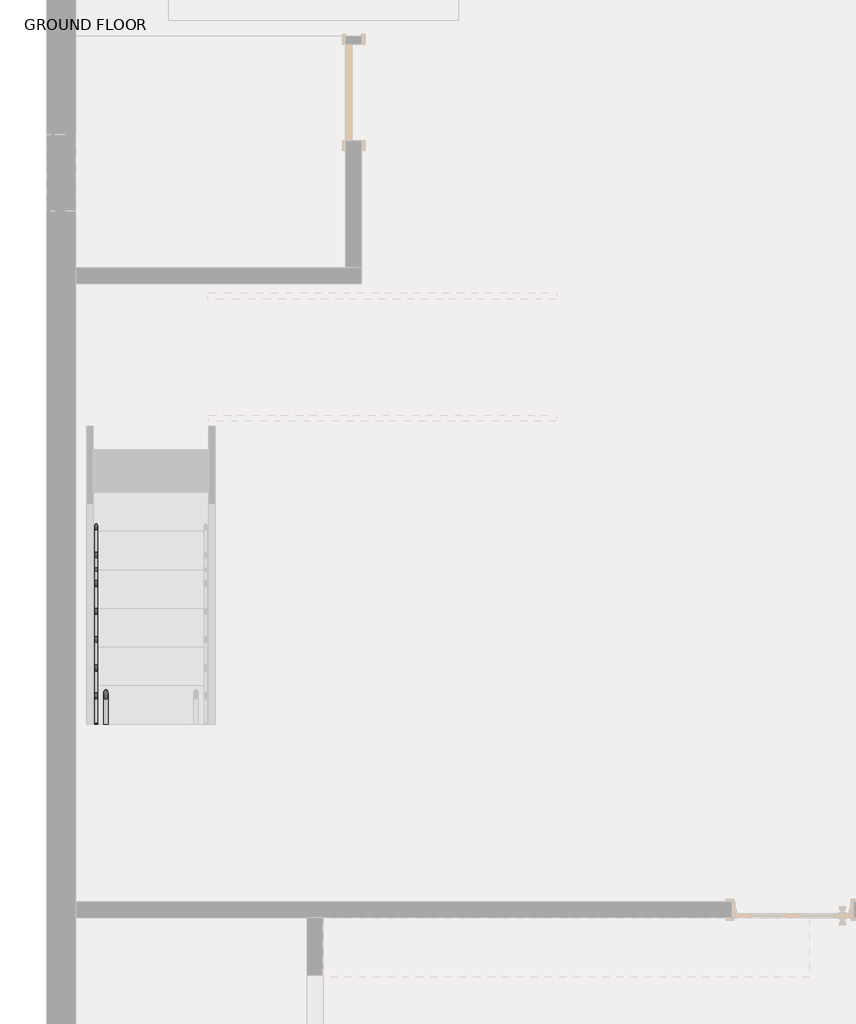
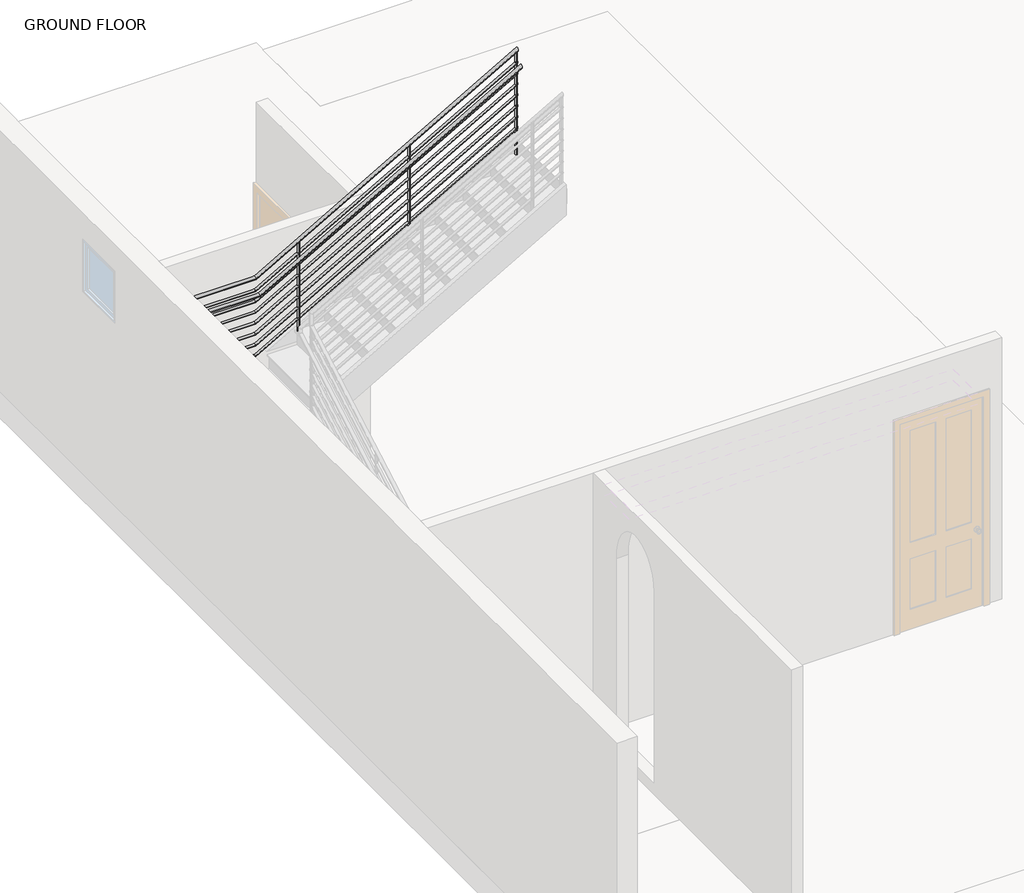
# One storey, part 2 of 3: 1 railing.
"""IFC4 building model written with IfcOpenShell, lengths in millimetres."""

from ifc_helpers import new_model, si_unit, point, frame, frame_2d, origin, place, context, project, spatial, circle_curve, ellipse_curve, trimmed, segment, composite_curve, outline, extrude, element, save
from ifc_brep_helpers import plane_surface, cylinder_surface, advanced_brep

model = new_model("IFC4")

# Units and contexts
model_context = context("Model", 3, world=origin())
ifc_project = project(units=[si_unit("LENGTHUNIT", "METRE", prefix="MILLI")], contexts=[model_context])

# Site, building, storey
site = spatial("IfcSite", under=ifc_project)
building = spatial("IfcBuilding", under=site)
storey = spatial("IfcBuildingStorey", under=building, Name="GROUND FLOOR", Elevation=304.8)

# Railing
placement = place(None, origin())
element("IfcRailing", 1, ObjectType="Guardrail - Pipe", at=placement, inside=storey, context=model_context, shape_type="SolidModel", body=[
    advanced_brep(
    [(-6821.0257327, 1771.427543, 1371.43057), (-6859.1257327, 1771.427543, 1371.43057), (-6821.0257327, 4367.2865455, 2854.7785714), (-6859.1257327, 4367.2865455, 2854.7785714), (-6821.0257327, 5003.577543, 2854.7785714), (-6859.1257327, 5041.677543, 2854.7785714), (-6174.6167301, 5003.577543, 2854.7785714), (-6174.6167301, 5041.677543, 2854.7785714), (-3284.0757327, 5003.577543, 4506.5162843), (-3284.0757327, 5041.677543, 4506.5162843)],
    [
        (0, 1, ellipse_curve(frame((-6840.0757327, 1771.427543, 1371.43057), z_axis=(0.0, -1.0, 0.0), x_axis=(0.0, 0.0, -1.0)), 21.9408586, 19.05)),
        (1, 0, ellipse_curve(frame((-6840.0757327, 1771.427543, 1371.43057), z_axis=(0.0, -1.0, 0.0), x_axis=(0.0, 0.0, -1.0)), 21.9408586, 19.05)),
        (0, 2),
        (2, 3, ellipse_curve(frame((-6840.0757327, 4367.2865455, 2854.7785714), z_axis=(0.0, -0.9664996487646668, -0.256667935157035), x_axis=(0.0, 0.2566679351570357, -0.9664996487646664)), 19.710302, 19.05)),
        (3, 1),
        (3, 2, ellipse_curve(frame((-6840.0757327, 4367.2865455, 2854.7785714), z_axis=(0.0, -0.9664996487646668, -0.256667935157035), x_axis=(0.0, 0.2566679351570357, -0.9664996487646664)), 19.710302, 19.05)),
        (2, 4),
        (4, 5, ellipse_curve(frame((-6840.0757327, 5022.627543, 2854.7785714), z_axis=(-0.7071067811865486, -0.7071067811865465, 0.0), x_axis=(0.7071067811865465, -0.7071067811865486, 0.0)), 26.9407684, 19.05)),
        (5, 3),
        (5, 4, ellipse_curve(frame((-6840.0757327, 5022.627543, 2854.7785714), z_axis=(-0.7071067811865486, -0.7071067811865465, 0.0), x_axis=(0.7071067811865465, -0.7071067811865486, 0.0)), 26.9407684, 19.05)),
        (4, 6),
        (6, 7, ellipse_curve(frame((-6174.6167301, 5022.627543, 2854.7785714), z_axis=(-0.9664996487646668, 0.0, -0.2566679351570351), x_axis=(-0.25666793515703434, 0.0, 0.9664996487646668)), 19.710302, 19.05)),
        (7, 5),
        (7, 6, ellipse_curve(frame((-6174.6167301, 5022.627543, 2854.7785714), z_axis=(-0.9664996487646668, 0.0, -0.2566679351570351), x_axis=(-0.25666793515703434, 0.0, 0.9664996487646668)), 19.710302, 19.05)),
        (8, 9, ellipse_curve(frame((-3284.0757327, 5022.627543, 4506.5162843), z_axis=(1.0, 0.0, 0.0), x_axis=(0.0, 0.0, -1.0)), 21.9408586, 19.05)),
        (9, 8, ellipse_curve(frame((-3284.0757327, 5022.627543, 4506.5162843), z_axis=(1.0, 0.0, 0.0), x_axis=(0.0, 0.0, -1.0)), 21.9408586, 19.05)),
        (6, 8),
        (9, 7),
    ],
    [
        plane_surface(frame((-6840.0757327, 1771.427543, 1393.3714286), z_axis=(0.0, -1.0, 0.0), x_axis=(0.0, 0.0, 1.0))),
        cylinder_surface(frame((-6840.0757327, 1780.8789898, 1376.8313967), z_axis=(0.0, -0.8682431421244483, -0.496138938356853), x_axis=(-1.0, 0.0, 0.0)), 19.05),
        cylinder_surface(frame((-6840.0757327, 4362.227543, 2854.7785714), z_axis=(0.0, -1.0, 0.0), x_axis=(-1.0, 0.0, 0.0)), 19.05),
        cylinder_surface(frame((-6840.0757327, 5022.627543, 2854.7785714), z_axis=(-1.0, 0.0, 0.0), x_axis=(0.0, 1.0, 0.0)), 19.05),
        plane_surface(frame((-3284.0757327, 5022.627543, 4528.4571429), z_axis=(1.0, 0.0, 0.0), x_axis=(0.0, 1.0, 0.0))),
        cylinder_surface(frame((-6170.2242859, 5022.627543, 2857.2885396), z_axis=(-0.8682431421244482, 0.0, -0.49613893835685324), x_axis=(0.0, 1.0, 0.0)), 19.05),
    ],
    [
        (0, [[1, 2]]),
        (1, [[-1, 3, 4, 5]]),
        (1, [[-2, -5, 6, -3]]),
        (2, [[-4, 7, 8, 9]]),
        (2, [[-6, -9, 10, -7]]),
        (3, [[-8, 11, 12, 13]]),
        (3, [[-10, -13, 14, -11]]),
        (4, [[15, 16]]),
        (5, [[-12, 17, -16, 18]]),
        (5, [[-14, -18, -15, -17]]),
    ],
),
    advanced_brep(
    [(-6897.2257327, 1771.427543, 1523.83057), (-6935.3257327, 1771.427543, 1523.83057), (-3284.0757327, 5079.777543, 4658.9162843), (-3284.0757327, 5117.877543, 4658.9162843), (-6897.2257327, 4367.2865455, 3007.1785714), (-6935.3257327, 4367.2865455, 3007.1785714), (-6897.2257327, 5079.777543, 3007.1785714), (-6935.3257327, 5117.877543, 3007.1785714), (-6174.6167301, 5079.777543, 3007.1785714), (-6174.6167301, 5117.877543, 3007.1785714)],
    [
        (0, 1, ellipse_curve(frame((-6916.2757327, 1771.427543, 1523.83057), z_axis=(0.0, -1.0, 0.0), x_axis=(0.0, 0.0, -1.0)), 21.9408586, 19.05)),
        (1, 0, ellipse_curve(frame((-6916.2757327, 1771.427543, 1523.83057), z_axis=(0.0, -1.0, 0.0), x_axis=(0.0, 0.0, -1.0)), 21.9408586, 19.05)),
        (2, 3, ellipse_curve(frame((-3284.0757327, 5098.827543, 4658.9162843), z_axis=(1.0, 0.0, 0.0), x_axis=(0.0, 0.0, -1.0)), 21.9408586, 19.05)),
        (3, 2, ellipse_curve(frame((-3284.0757327, 5098.827543, 4658.9162843), z_axis=(1.0, 0.0, 0.0), x_axis=(0.0, 0.0, -1.0)), 21.9408586, 19.05)),
        (0, 4),
        (4, 5, ellipse_curve(frame((-6916.2757327, 4367.2865455, 3007.1785714), z_axis=(0.0, -0.9664996487646668, -0.256667935157035), x_axis=(0.0, 0.2566679351570357, -0.9664996487646664)), 19.710302, 19.05)),
        (5, 1),
        (5, 4, ellipse_curve(frame((-6916.2757327, 4367.2865455, 3007.1785714), z_axis=(0.0, -0.9664996487646668, -0.256667935157035), x_axis=(0.0, 0.2566679351570357, -0.9664996487646664)), 19.710302, 19.05)),
        (4, 6),
        (6, 7, ellipse_curve(frame((-6916.2757327, 5098.827543, 3007.1785714), z_axis=(-0.7071067811865487, -0.7071067811865464, 0.0), x_axis=(0.7071067811865464, -0.7071067811865487, 0.0)), 26.9407684, 19.05)),
        (7, 5),
        (7, 6, ellipse_curve(frame((-6916.2757327, 5098.827543, 3007.1785714), z_axis=(-0.7071067811865487, -0.7071067811865464, 0.0), x_axis=(0.7071067811865464, -0.7071067811865487, 0.0)), 26.9407684, 19.05)),
        (6, 8),
        (8, 9, ellipse_curve(frame((-6174.6167301, 5098.827543, 3007.1785714), z_axis=(-0.9664996487646668, 0.0, -0.2566679351570351), x_axis=(-0.25666793515703434, 0.0, 0.9664996487646668)), 19.710302, 19.05)),
        (9, 7),
        (9, 8, ellipse_curve(frame((-6174.6167301, 5098.827543, 3007.1785714), z_axis=(-0.9664996487646668, 0.0, -0.2566679351570351), x_axis=(-0.25666793515703434, 0.0, 0.9664996487646668)), 19.710302, 19.05)),
        (8, 2),
        (3, 9),
    ],
    [
        plane_surface(frame((-6916.2757327, 1771.427543, 1545.7714286), z_axis=(0.0, -1.0, 0.0), x_axis=(0.0, 0.0, 1.0))),
        plane_surface(frame((-3284.0757327, 5098.827543, 4680.8571429), z_axis=(1.0, 0.0, 0.0), x_axis=(0.0, 1.0, 0.0))),
        cylinder_surface(frame((-6916.2757327, 1780.8789898, 1529.2313967), z_axis=(0.0, -0.8682431421244483, -0.496138938356853), x_axis=(-1.0, 0.0, 0.0)), 19.05),
        cylinder_surface(frame((-6916.2757327, 4362.227543, 3007.1785714), z_axis=(0.0, -1.0, 0.0), x_axis=(-1.0, 0.0, 0.0)), 19.05),
        cylinder_surface(frame((-6916.2757327, 5098.827543, 3007.1785714), z_axis=(-1.0, 0.0, 0.0), x_axis=(0.0, 1.0, 0.0)), 19.05),
        cylinder_surface(frame((-6170.2242859, 5098.827543, 3009.6885396), z_axis=(-0.8682431421244482, 0.0, -0.49613893835685324), x_axis=(0.0, 1.0, 0.0)), 19.05),
    ],
    [
        (0, [[1, 2]]),
        (1, [[3, 4]]),
        (2, [[-1, 5, 6, 7]]),
        (2, [[-2, -7, 8, -5]]),
        (3, [[-6, 9, 10, 11]]),
        (3, [[-8, -11, 12, -9]]),
        (4, [[-10, 13, 14, 15]]),
        (4, [[-12, -15, 16, -13]]),
        (5, [[-14, 17, -4, 18]]),
        (5, [[-16, -18, -3, -17]]),
    ],
),
    advanced_brep(
    [(-6903.5757327, 1771.427543, 1378.7441895), (-6928.9757327, 1771.427543, 1378.7441895), (-6903.5757327, 4365.6002113, 2861.1285714), (-6928.9757327, 4365.6002113, 2861.1285714), (-6903.5757327, 5086.127543, 2861.1285714), (-6928.9757327, 5086.127543, 2861.1285714)],
    [
        (0, 1, ellipse_curve(frame((-6916.2757327, 1771.427543, 1378.7441895), z_axis=(0.0, -1.0, 0.0), x_axis=(0.0, 0.0, -1.0)), 14.6272391, 12.7)),
        (1, 0, ellipse_curve(frame((-6916.2757327, 1771.427543, 1378.7441895), z_axis=(0.0, -1.0, 0.0), x_axis=(0.0, 0.0, -1.0)), 14.6272391, 12.7)),
        (0, 2),
        (2, 3, ellipse_curve(frame((-6916.2757327, 4365.6002113, 2861.1285714), z_axis=(0.0, -0.9664996487646668, -0.256667935157035), x_axis=(0.0, 0.2566679351570357, -0.9664996487646664)), 13.1402014, 12.7)),
        (3, 1),
        (3, 2, ellipse_curve(frame((-6916.2757327, 4365.6002113, 2861.1285714), z_axis=(0.0, -0.9664996487646668, -0.256667935157035), x_axis=(0.0, 0.2566679351570357, -0.9664996487646664)), 13.1402014, 12.7)),
        (4, 5, circle_curve(frame((-6916.2757327, 5086.127543, 2861.1285714), z_axis=(0.0, 1.0, 0.0), x_axis=(-1.0, 0.0, 0.0)), 12.7)),
        (5, 4, circle_curve(frame((-6916.2757327, 5086.127543, 2861.1285714), z_axis=(0.0, 1.0, 0.0), x_axis=(-1.0, 0.0, 0.0)), 12.7)),
        (2, 4),
        (5, 3),
    ],
    [
        plane_surface(frame((-6916.2757327, 1771.427543, 1393.3714286), z_axis=(0.0, -1.0, 0.0), x_axis=(0.0, 0.0, 1.0))),
        cylinder_surface(frame((-6916.2757327, 1777.7285075, 1382.3447407), z_axis=(0.0, -0.8682431421244483, -0.496138938356853), x_axis=(-1.0, 0.0, 0.0)), 12.7),
        plane_surface(frame((-6916.2757327, 5086.127543, 2873.8285714), z_axis=(0.0, 1.0, 0.0), x_axis=(0.0, 0.0, 1.0))),
        cylinder_surface(frame((-6916.2757327, 4362.227543, 2861.1285714), z_axis=(0.0, -1.0, 0.0), x_axis=(-1.0, 0.0, 0.0)), 12.7),
    ],
    [
        (0, [[1, 2]]),
        (1, [[-1, 3, 4, 5]]),
        (1, [[-2, -5, 6, -3]]),
        (2, [[7, 8]]),
        (3, [[-4, 9, -8, 10]]),
        (3, [[-6, -10, -7, -9]]),
    ],
),
    advanced_brep(
    [(-6928.9757327, 5086.127543, 2861.1285714), (-6928.9757327, 5111.527543, 2861.1285714), (-6176.3030643, 5086.127543, 2861.1285714), (-6176.3030643, 5111.527543, 2861.1285714), (-3284.0757327, 5086.127543, 4513.8299038), (-3284.0757327, 5111.527543, 4513.8299038)],
    [
        (0, 1, circle_curve(frame((-6928.9757327, 5098.827543, 2861.1285714), z_axis=(-1.0, 0.0, 0.0), x_axis=(0.0, 1.0, 0.0)), 12.7)),
        (1, 0, circle_curve(frame((-6928.9757327, 5098.827543, 2861.1285714), z_axis=(-1.0, 0.0, 0.0), x_axis=(0.0, 1.0, 0.0)), 12.7)),
        (0, 2),
        (2, 3, ellipse_curve(frame((-6176.3030643, 5098.827543, 2861.1285714), z_axis=(-0.9664996487646668, 0.0, -0.2566679351570349), x_axis=(-0.2566679351570344, 0.0, 0.9664996487646668)), 13.1402014, 12.7)),
        (3, 1),
        (3, 2, ellipse_curve(frame((-6176.3030643, 5098.827543, 2861.1285714), z_axis=(-0.9664996487646668, 0.0, -0.2566679351570349), x_axis=(-0.2566679351570344, 0.0, 0.9664996487646668)), 13.1402014, 12.7)),
        (4, 5, ellipse_curve(frame((-3284.0757327, 5098.827543, 4513.8299038), z_axis=(1.0, 0.0, 0.0), x_axis=(0.0, 0.0, -1.0)), 14.6272391, 12.7)),
        (5, 4, ellipse_curve(frame((-3284.0757327, 5098.827543, 4513.8299038), z_axis=(1.0, 0.0, 0.0), x_axis=(0.0, 0.0, -1.0)), 14.6272391, 12.7)),
        (2, 4),
        (5, 3),
    ],
    [
        plane_surface(frame((-6928.9757327, 5098.827543, 2873.8285714), z_axis=(-1.0, 0.0, 0.0), x_axis=(0.0, 1.0, 0.0))),
        cylinder_surface(frame((-6928.9757327, 5098.827543, 2861.1285714), z_axis=(-1.0, 0.0, 0.0), x_axis=(0.0, 1.0, 0.0)), 12.7),
        plane_surface(frame((-3284.0757327, 5098.827543, 4528.4571429), z_axis=(1.0, 0.0, 0.0), x_axis=(0.0, 1.0, 0.0))),
        cylinder_surface(frame((-6173.3747682, 5098.827543, 2862.8018835), z_axis=(-0.8682431421244482, 0.0, -0.496138938356853), x_axis=(0.0, 1.0, 0.0)), 12.7),
    ],
    [
        (0, [[1, 2]]),
        (1, [[-1, 3, 4, 5]]),
        (1, [[-2, -5, 6, -3]]),
        (2, [[7, 8]]),
        (3, [[-4, 9, -8, 10]]),
        (3, [[-6, -10, -7, -9]]),
    ],
),
    advanced_brep(
    [(-6903.5757327, 1771.427543, 1251.7441895), (-6928.9757327, 1771.427543, 1251.7441895), (-6903.5757327, 4365.6002113, 2734.1285714), (-6928.9757327, 4365.6002113, 2734.1285714), (-6903.5757327, 5086.127543, 2734.1285714), (-6928.9757327, 5086.127543, 2734.1285714)],
    [
        (0, 1, ellipse_curve(frame((-6916.2757327, 1771.427543, 1251.7441895), z_axis=(0.0, -1.0, 0.0), x_axis=(0.0, 0.0, -1.0)), 14.6272391, 12.7)),
        (1, 0, ellipse_curve(frame((-6916.2757327, 1771.427543, 1251.7441895), z_axis=(0.0, -1.0, 0.0), x_axis=(0.0, 0.0, -1.0)), 14.6272391, 12.7)),
        (0, 2),
        (2, 3, ellipse_curve(frame((-6916.2757327, 4365.6002113, 2734.1285714), z_axis=(0.0, -0.9664996487646668, -0.256667935157035), x_axis=(0.0, 0.2566679351570357, -0.9664996487646664)), 13.1402014, 12.7)),
        (3, 1),
        (3, 2, ellipse_curve(frame((-6916.2757327, 4365.6002113, 2734.1285714), z_axis=(0.0, -0.9664996487646668, -0.256667935157035), x_axis=(0.0, 0.2566679351570357, -0.9664996487646664)), 13.1402014, 12.7)),
        (4, 5, circle_curve(frame((-6916.2757327, 5086.127543, 2734.1285714), z_axis=(0.0, 1.0, 0.0), x_axis=(-1.0, 0.0, 0.0)), 12.7)),
        (5, 4, circle_curve(frame((-6916.2757327, 5086.127543, 2734.1285714), z_axis=(0.0, 1.0, 0.0), x_axis=(-1.0, 0.0, 0.0)), 12.7)),
        (2, 4),
        (5, 3),
    ],
    [
        plane_surface(frame((-6916.2757327, 1771.427543, 1266.3714286), z_axis=(0.0, -1.0, 0.0), x_axis=(0.0, 0.0, 1.0))),
        cylinder_surface(frame((-6916.2757327, 1777.7285075, 1255.3447407), z_axis=(0.0, -0.8682431421244483, -0.496138938356853), x_axis=(-1.0, 0.0, 0.0)), 12.7),
        plane_surface(frame((-6916.2757327, 5086.127543, 2746.8285714), z_axis=(0.0, 1.0, 0.0), x_axis=(0.0, 0.0, 1.0))),
        cylinder_surface(frame((-6916.2757327, 4362.227543, 2734.1285714), z_axis=(0.0, -1.0, 0.0), x_axis=(-1.0, 0.0, 0.0)), 12.7),
    ],
    [
        (0, [[1, 2]]),
        (1, [[-1, 3, 4, 5]]),
        (1, [[-2, -5, 6, -3]]),
        (2, [[7, 8]]),
        (3, [[-4, 9, -8, 10]]),
        (3, [[-6, -10, -7, -9]]),
    ],
),
    advanced_brep(
    [(-6928.9757327, 5086.127543, 2734.1285714), (-6928.9757327, 5111.527543, 2734.1285714), (-6176.3030643, 5086.127543, 2734.1285714), (-6176.3030643, 5111.527543, 2734.1285714), (-3284.0757327, 5086.127543, 4386.8299038), (-3284.0757327, 5111.527543, 4386.8299038)],
    [
        (0, 1, circle_curve(frame((-6928.9757327, 5098.827543, 2734.1285714), z_axis=(-1.0, 0.0, 0.0), x_axis=(0.0, 1.0, 0.0)), 12.7)),
        (1, 0, circle_curve(frame((-6928.9757327, 5098.827543, 2734.1285714), z_axis=(-1.0, 0.0, 0.0), x_axis=(0.0, 1.0, 0.0)), 12.7)),
        (0, 2),
        (2, 3, ellipse_curve(frame((-6176.3030643, 5098.827543, 2734.1285714), z_axis=(-0.9664996487646668, 0.0, -0.2566679351570349), x_axis=(-0.2566679351570344, 0.0, 0.9664996487646668)), 13.1402014, 12.7)),
        (3, 1),
        (3, 2, ellipse_curve(frame((-6176.3030643, 5098.827543, 2734.1285714), z_axis=(-0.9664996487646668, 0.0, -0.2566679351570349), x_axis=(-0.2566679351570344, 0.0, 0.9664996487646668)), 13.1402014, 12.7)),
        (4, 5, ellipse_curve(frame((-3284.0757327, 5098.827543, 4386.8299038), z_axis=(1.0, 0.0, 0.0), x_axis=(0.0, 0.0, -1.0)), 14.6272391, 12.7)),
        (5, 4, ellipse_curve(frame((-3284.0757327, 5098.827543, 4386.8299038), z_axis=(1.0, 0.0, 0.0), x_axis=(0.0, 0.0, -1.0)), 14.6272391, 12.7)),
        (2, 4),
        (5, 3),
    ],
    [
        plane_surface(frame((-6928.9757327, 5098.827543, 2746.8285714), z_axis=(-1.0, 0.0, 0.0), x_axis=(0.0, 1.0, 0.0))),
        cylinder_surface(frame((-6928.9757327, 5098.827543, 2734.1285714), z_axis=(-1.0, 0.0, 0.0), x_axis=(0.0, 1.0, 0.0)), 12.7),
        plane_surface(frame((-3284.0757327, 5098.827543, 4401.4571429), z_axis=(1.0, 0.0, 0.0), x_axis=(0.0, 1.0, 0.0))),
        cylinder_surface(frame((-6173.3747682, 5098.827543, 2735.8018835), z_axis=(-0.8682431421244482, 0.0, -0.496138938356853), x_axis=(0.0, 1.0, 0.0)), 12.7),
    ],
    [
        (0, [[1, 2]]),
        (1, [[-1, 3, 4, 5]]),
        (1, [[-2, -5, 6, -3]]),
        (2, [[7, 8]]),
        (3, [[-4, 9, -8, 10]]),
        (3, [[-6, -10, -7, -9]]),
    ],
),
    advanced_brep(
    [(-6903.5757327, 1771.427543, 1124.7441895), (-6928.9757327, 1771.427543, 1124.7441895), (-6903.5757327, 4365.6002113, 2607.1285714), (-6928.9757327, 4365.6002113, 2607.1285714), (-6903.5757327, 5086.127543, 2607.1285714), (-6928.9757327, 5086.127543, 2607.1285714)],
    [
        (0, 1, ellipse_curve(frame((-6916.2757327, 1771.427543, 1124.7441895), z_axis=(0.0, -1.0, 0.0), x_axis=(0.0, 0.0, -1.0)), 14.6272391, 12.7)),
        (1, 0, ellipse_curve(frame((-6916.2757327, 1771.427543, 1124.7441895), z_axis=(0.0, -1.0, 0.0), x_axis=(0.0, 0.0, -1.0)), 14.6272391, 12.7)),
        (0, 2),
        (2, 3, ellipse_curve(frame((-6916.2757327, 4365.6002113, 2607.1285714), z_axis=(0.0, -0.9664996487646668, -0.256667935157035), x_axis=(0.0, 0.2566679351570357, -0.9664996487646664)), 13.1402014, 12.7)),
        (3, 1),
        (3, 2, ellipse_curve(frame((-6916.2757327, 4365.6002113, 2607.1285714), z_axis=(0.0, -0.9664996487646668, -0.256667935157035), x_axis=(0.0, 0.2566679351570357, -0.9664996487646664)), 13.1402014, 12.7)),
        (4, 5, circle_curve(frame((-6916.2757327, 5086.127543, 2607.1285714), z_axis=(0.0, 1.0, 0.0), x_axis=(-1.0, 0.0, 0.0)), 12.7)),
        (5, 4, circle_curve(frame((-6916.2757327, 5086.127543, 2607.1285714), z_axis=(0.0, 1.0, 0.0), x_axis=(-1.0, 0.0, 0.0)), 12.7)),
        (2, 4),
        (5, 3),
    ],
    [
        plane_surface(frame((-6916.2757327, 1771.427543, 1139.3714286), z_axis=(0.0, -1.0, 0.0), x_axis=(0.0, 0.0, 1.0))),
        cylinder_surface(frame((-6916.2757327, 1777.7285075, 1128.3447407), z_axis=(0.0, -0.8682431421244483, -0.496138938356853), x_axis=(-1.0, 0.0, 0.0)), 12.7),
        plane_surface(frame((-6916.2757327, 5086.127543, 2619.8285714), z_axis=(0.0, 1.0, 0.0), x_axis=(0.0, 0.0, 1.0))),
        cylinder_surface(frame((-6916.2757327, 4362.227543, 2607.1285714), z_axis=(0.0, -1.0, 0.0), x_axis=(-1.0, 0.0, 0.0)), 12.7),
    ],
    [
        (0, [[1, 2]]),
        (1, [[-1, 3, 4, 5]]),
        (1, [[-2, -5, 6, -3]]),
        (2, [[7, 8]]),
        (3, [[-4, 9, -8, 10]]),
        (3, [[-6, -10, -7, -9]]),
    ],
),
    advanced_brep(
    [(-6928.9757327, 5086.127543, 2607.1285714), (-6928.9757327, 5111.527543, 2607.1285714), (-6176.3030643, 5086.127543, 2607.1285714), (-6176.3030643, 5111.527543, 2607.1285714), (-3284.0757327, 5086.127543, 4259.8299038), (-3284.0757327, 5111.527543, 4259.8299038)],
    [
        (0, 1, circle_curve(frame((-6928.9757327, 5098.827543, 2607.1285714), z_axis=(-1.0, 0.0, 0.0), x_axis=(0.0, 1.0, 0.0)), 12.7)),
        (1, 0, circle_curve(frame((-6928.9757327, 5098.827543, 2607.1285714), z_axis=(-1.0, 0.0, 0.0), x_axis=(0.0, 1.0, 0.0)), 12.7)),
        (0, 2),
        (2, 3, ellipse_curve(frame((-6176.3030643, 5098.827543, 2607.1285714), z_axis=(-0.9664996487646668, 0.0, -0.2566679351570349), x_axis=(-0.2566679351570344, 0.0, 0.9664996487646668)), 13.1402014, 12.7)),
        (3, 1),
        (3, 2, ellipse_curve(frame((-6176.3030643, 5098.827543, 2607.1285714), z_axis=(-0.9664996487646668, 0.0, -0.2566679351570349), x_axis=(-0.2566679351570344, 0.0, 0.9664996487646668)), 13.1402014, 12.7)),
        (4, 5, ellipse_curve(frame((-3284.0757327, 5098.827543, 4259.8299038), z_axis=(1.0, 0.0, 0.0), x_axis=(0.0, 0.0, -1.0)), 14.6272391, 12.7)),
        (5, 4, ellipse_curve(frame((-3284.0757327, 5098.827543, 4259.8299038), z_axis=(1.0, 0.0, 0.0), x_axis=(0.0, 0.0, -1.0)), 14.6272391, 12.7)),
        (2, 4),
        (5, 3),
    ],
    [
        plane_surface(frame((-6928.9757327, 5098.827543, 2619.8285714), z_axis=(-1.0, 0.0, 0.0), x_axis=(0.0, 1.0, 0.0))),
        cylinder_surface(frame((-6928.9757327, 5098.827543, 2607.1285714), z_axis=(-1.0, 0.0, 0.0), x_axis=(0.0, 1.0, 0.0)), 12.7),
        plane_surface(frame((-3284.0757327, 5098.827543, 4274.4571429), z_axis=(1.0, 0.0, 0.0), x_axis=(0.0, 1.0, 0.0))),
        cylinder_surface(frame((-6173.3747682, 5098.827543, 2608.8018835), z_axis=(-0.8682431421244482, 0.0, -0.496138938356853), x_axis=(0.0, 1.0, 0.0)), 12.7),
    ],
    [
        (0, [[1, 2]]),
        (1, [[-1, 3, 4, 5]]),
        (1, [[-2, -5, 6, -3]]),
        (2, [[7, 8]]),
        (3, [[-4, 9, -8, 10]]),
        (3, [[-6, -10, -7, -9]]),
    ],
),
    advanced_brep(
    [(-6903.5757327, 1771.427543, 997.7441895), (-6928.9757327, 1771.427543, 997.7441895), (-6903.5757327, 4365.6002113, 2480.1285714), (-6928.9757327, 4365.6002113, 2480.1285714), (-6903.5757327, 5086.127543, 2480.1285714), (-6928.9757327, 5086.127543, 2480.1285714)],
    [
        (0, 1, ellipse_curve(frame((-6916.2757327, 1771.427543, 997.7441895), z_axis=(0.0, -1.0, 0.0), x_axis=(0.0, 0.0, -1.0)), 14.6272391, 12.7)),
        (1, 0, ellipse_curve(frame((-6916.2757327, 1771.427543, 997.7441895), z_axis=(0.0, -1.0, 0.0), x_axis=(0.0, 0.0, -1.0)), 14.6272391, 12.7)),
        (0, 2),
        (2, 3, ellipse_curve(frame((-6916.2757327, 4365.6002113, 2480.1285714), z_axis=(0.0, -0.9664996487646668, -0.256667935157035), x_axis=(0.0, 0.2566679351570357, -0.9664996487646664)), 13.1402014, 12.7)),
        (3, 1),
        (3, 2, ellipse_curve(frame((-6916.2757327, 4365.6002113, 2480.1285714), z_axis=(0.0, -0.9664996487646668, -0.256667935157035), x_axis=(0.0, 0.2566679351570357, -0.9664996487646664)), 13.1402014, 12.7)),
        (4, 5, circle_curve(frame((-6916.2757327, 5086.127543, 2480.1285714), z_axis=(0.0, 1.0, 0.0), x_axis=(-1.0, 0.0, 0.0)), 12.7)),
        (5, 4, circle_curve(frame((-6916.2757327, 5086.127543, 2480.1285714), z_axis=(0.0, 1.0, 0.0), x_axis=(-1.0, 0.0, 0.0)), 12.7)),
        (2, 4),
        (5, 3),
    ],
    [
        plane_surface(frame((-6916.2757327, 1771.427543, 1012.3714286), z_axis=(0.0, -1.0, 0.0), x_axis=(0.0, 0.0, 1.0))),
        cylinder_surface(frame((-6916.2757327, 1777.7285075, 1001.3447407), z_axis=(0.0, -0.8682431421244483, -0.496138938356853), x_axis=(-1.0, 0.0, 0.0)), 12.7),
        plane_surface(frame((-6916.2757327, 5086.127543, 2492.8285714), z_axis=(0.0, 1.0, 0.0), x_axis=(0.0, 0.0, 1.0))),
        cylinder_surface(frame((-6916.2757327, 4362.227543, 2480.1285714), z_axis=(0.0, -1.0, 0.0), x_axis=(-1.0, 0.0, 0.0)), 12.7),
    ],
    [
        (0, [[1, 2]]),
        (1, [[-1, 3, 4, 5]]),
        (1, [[-2, -5, 6, -3]]),
        (2, [[7, 8]]),
        (3, [[-4, 9, -8, 10]]),
        (3, [[-6, -10, -7, -9]]),
    ],
),
    advanced_brep(
    [(-6928.9757327, 5086.127543, 2480.1285714), (-6928.9757327, 5111.527543, 2480.1285714), (-6176.3030643, 5086.127543, 2480.1285714), (-6176.3030643, 5111.527543, 2480.1285714), (-3284.0757327, 5086.127543, 4132.8299038), (-3284.0757327, 5111.527543, 4132.8299038)],
    [
        (0, 1, circle_curve(frame((-6928.9757327, 5098.827543, 2480.1285714), z_axis=(-1.0, 0.0, 0.0), x_axis=(0.0, 1.0, 0.0)), 12.7)),
        (1, 0, circle_curve(frame((-6928.9757327, 5098.827543, 2480.1285714), z_axis=(-1.0, 0.0, 0.0), x_axis=(0.0, 1.0, 0.0)), 12.7)),
        (0, 2),
        (2, 3, ellipse_curve(frame((-6176.3030643, 5098.827543, 2480.1285714), z_axis=(-0.9664996487646668, 0.0, -0.2566679351570349), x_axis=(-0.2566679351570344, 0.0, 0.9664996487646668)), 13.1402014, 12.7)),
        (3, 1),
        (3, 2, ellipse_curve(frame((-6176.3030643, 5098.827543, 2480.1285714), z_axis=(-0.9664996487646668, 0.0, -0.2566679351570349), x_axis=(-0.2566679351570344, 0.0, 0.9664996487646668)), 13.1402014, 12.7)),
        (4, 5, ellipse_curve(frame((-3284.0757327, 5098.827543, 4132.8299038), z_axis=(1.0, 0.0, 0.0), x_axis=(0.0, 0.0, -1.0)), 14.6272391, 12.7)),
        (5, 4, ellipse_curve(frame((-3284.0757327, 5098.827543, 4132.8299038), z_axis=(1.0, 0.0, 0.0), x_axis=(0.0, 0.0, -1.0)), 14.6272391, 12.7)),
        (2, 4),
        (5, 3),
    ],
    [
        plane_surface(frame((-6928.9757327, 5098.827543, 2492.8285714), z_axis=(-1.0, 0.0, 0.0), x_axis=(0.0, 1.0, 0.0))),
        cylinder_surface(frame((-6928.9757327, 5098.827543, 2480.1285714), z_axis=(-1.0, 0.0, 0.0), x_axis=(0.0, 1.0, 0.0)), 12.7),
        plane_surface(frame((-3284.0757327, 5098.827543, 4147.4571429), z_axis=(1.0, 0.0, 0.0), x_axis=(0.0, 1.0, 0.0))),
        cylinder_surface(frame((-6173.3747682, 5098.827543, 2481.8018835), z_axis=(-0.8682431421244482, 0.0, -0.496138938356853), x_axis=(0.0, 1.0, 0.0)), 12.7),
    ],
    [
        (0, [[1, 2]]),
        (1, [[-1, 3, 4, 5]]),
        (1, [[-2, -5, 6, -3]]),
        (2, [[7, 8]]),
        (3, [[-4, 9, -8, 10]]),
        (3, [[-6, -10, -7, -9]]),
    ],
),
    advanced_brep(
    [(-6903.5757327, 1771.427543, 870.7441895), (-6928.9757327, 1771.427543, 870.7441895), (-6903.5757327, 4365.6002113, 2353.1285714), (-6928.9757327, 4365.6002113, 2353.1285714), (-6903.5757327, 5086.127543, 2353.1285714), (-6928.9757327, 5086.127543, 2353.1285714)],
    [
        (0, 1, ellipse_curve(frame((-6916.2757327, 1771.427543, 870.7441895), z_axis=(0.0, -1.0, 0.0), x_axis=(0.0, 0.0, -1.0)), 14.6272391, 12.7)),
        (1, 0, ellipse_curve(frame((-6916.2757327, 1771.427543, 870.7441895), z_axis=(0.0, -1.0, 0.0), x_axis=(0.0, 0.0, -1.0)), 14.6272391, 12.7)),
        (0, 2),
        (2, 3, ellipse_curve(frame((-6916.2757327, 4365.6002113, 2353.1285714), z_axis=(0.0, -0.9664996487646668, -0.256667935157035), x_axis=(0.0, 0.2566679351570357, -0.9664996487646664)), 13.1402014, 12.7)),
        (3, 1),
        (3, 2, ellipse_curve(frame((-6916.2757327, 4365.6002113, 2353.1285714), z_axis=(0.0, -0.9664996487646668, -0.256667935157035), x_axis=(0.0, 0.2566679351570357, -0.9664996487646664)), 13.1402014, 12.7)),
        (4, 5, circle_curve(frame((-6916.2757327, 5086.127543, 2353.1285714), z_axis=(0.0, 1.0, 0.0), x_axis=(-1.0, 0.0, 0.0)), 12.7)),
        (5, 4, circle_curve(frame((-6916.2757327, 5086.127543, 2353.1285714), z_axis=(0.0, 1.0, 0.0), x_axis=(-1.0, 0.0, 0.0)), 12.7)),
        (2, 4),
        (5, 3),
    ],
    [
        plane_surface(frame((-6916.2757327, 1771.427543, 885.3714286), z_axis=(0.0, -1.0, 0.0), x_axis=(0.0, 0.0, 1.0))),
        cylinder_surface(frame((-6916.2757327, 1777.7285075, 874.3447407), z_axis=(0.0, -0.8682431421244483, -0.496138938356853), x_axis=(-1.0, 0.0, 0.0)), 12.7),
        plane_surface(frame((-6916.2757327, 5086.127543, 2365.8285714), z_axis=(0.0, 1.0, 0.0), x_axis=(0.0, 0.0, 1.0))),
        cylinder_surface(frame((-6916.2757327, 4362.227543, 2353.1285714), z_axis=(0.0, -1.0, 0.0), x_axis=(-1.0, 0.0, 0.0)), 12.7),
    ],
    [
        (0, [[1, 2]]),
        (1, [[-1, 3, 4, 5]]),
        (1, [[-2, -5, 6, -3]]),
        (2, [[7, 8]]),
        (3, [[-4, 9, -8, 10]]),
        (3, [[-6, -10, -7, -9]]),
    ],
),
    advanced_brep(
    [(-6928.9757327, 5086.127543, 2353.1285714), (-6928.9757327, 5111.527543, 2353.1285714), (-6176.3030643, 5086.127543, 2353.1285714), (-6176.3030643, 5111.527543, 2353.1285714), (-3284.0757327, 5086.127543, 4005.8299038), (-3284.0757327, 5111.527543, 4005.8299038)],
    [
        (0, 1, circle_curve(frame((-6928.9757327, 5098.827543, 2353.1285714), z_axis=(-1.0, 0.0, 0.0), x_axis=(0.0, 1.0, 0.0)), 12.7)),
        (1, 0, circle_curve(frame((-6928.9757327, 5098.827543, 2353.1285714), z_axis=(-1.0, 0.0, 0.0), x_axis=(0.0, 1.0, 0.0)), 12.7)),
        (0, 2),
        (2, 3, ellipse_curve(frame((-6176.3030643, 5098.827543, 2353.1285714), z_axis=(-0.9664996487646668, 0.0, -0.2566679351570349), x_axis=(-0.2566679351570344, 0.0, 0.9664996487646668)), 13.1402014, 12.7)),
        (3, 1),
        (3, 2, ellipse_curve(frame((-6176.3030643, 5098.827543, 2353.1285714), z_axis=(-0.9664996487646668, 0.0, -0.2566679351570349), x_axis=(-0.2566679351570344, 0.0, 0.9664996487646668)), 13.1402014, 12.7)),
        (4, 5, ellipse_curve(frame((-3284.0757327, 5098.827543, 4005.8299038), z_axis=(1.0, 0.0, 0.0), x_axis=(0.0, 0.0, -1.0)), 14.6272391, 12.7)),
        (5, 4, ellipse_curve(frame((-3284.0757327, 5098.827543, 4005.8299038), z_axis=(1.0, 0.0, 0.0), x_axis=(0.0, 0.0, -1.0)), 14.6272391, 12.7)),
        (2, 4),
        (5, 3),
    ],
    [
        plane_surface(frame((-6928.9757327, 5098.827543, 2365.8285714), z_axis=(-1.0, 0.0, 0.0), x_axis=(0.0, 1.0, 0.0))),
        cylinder_surface(frame((-6928.9757327, 5098.827543, 2353.1285714), z_axis=(-1.0, 0.0, 0.0), x_axis=(0.0, 1.0, 0.0)), 12.7),
        plane_surface(frame((-3284.0757327, 5098.827543, 4020.4571429), z_axis=(1.0, 0.0, 0.0), x_axis=(0.0, 1.0, 0.0))),
        cylinder_surface(frame((-6173.3747682, 5098.827543, 2354.8018835), z_axis=(-0.8682431421244482, 0.0, -0.496138938356853), x_axis=(0.0, 1.0, 0.0)), 12.7),
    ],
    [
        (0, [[1, 2]]),
        (1, [[-1, 3, 4, 5]]),
        (1, [[-2, -5, 6, -3]]),
        (2, [[7, 8]]),
        (3, [[-4, 9, -8, 10]]),
        (3, [[-6, -10, -7, -9]]),
    ],
),
    advanced_brep(
    [(-6903.5757327, 1771.427543, 743.7441895), (-6928.9757327, 1771.427543, 743.7441895), (-6903.5757327, 4365.6002113, 2226.1285714), (-6928.9757327, 4365.6002113, 2226.1285714), (-6903.5757327, 5086.127543, 2226.1285714), (-6928.9757327, 5086.127543, 2226.1285714)],
    [
        (0, 1, ellipse_curve(frame((-6916.2757327, 1771.427543, 743.7441895), z_axis=(0.0, -1.0, 0.0), x_axis=(0.0, 0.0, -1.0)), 14.6272391, 12.7)),
        (1, 0, ellipse_curve(frame((-6916.2757327, 1771.427543, 743.7441895), z_axis=(0.0, -1.0, 0.0), x_axis=(0.0, 0.0, -1.0)), 14.6272391, 12.7)),
        (0, 2),
        (2, 3, ellipse_curve(frame((-6916.2757327, 4365.6002113, 2226.1285714), z_axis=(0.0, -0.9664996487646668, -0.256667935157035), x_axis=(0.0, 0.2566679351570357, -0.9664996487646664)), 13.1402014, 12.7)),
        (3, 1),
        (3, 2, ellipse_curve(frame((-6916.2757327, 4365.6002113, 2226.1285714), z_axis=(0.0, -0.9664996487646668, -0.256667935157035), x_axis=(0.0, 0.2566679351570357, -0.9664996487646664)), 13.1402014, 12.7)),
        (4, 5, circle_curve(frame((-6916.2757327, 5086.127543, 2226.1285714), z_axis=(0.0, 1.0, 0.0), x_axis=(-1.0, 0.0, 0.0)), 12.7)),
        (5, 4, circle_curve(frame((-6916.2757327, 5086.127543, 2226.1285714), z_axis=(0.0, 1.0, 0.0), x_axis=(-1.0, 0.0, 0.0)), 12.7)),
        (2, 4),
        (5, 3),
    ],
    [
        plane_surface(frame((-6916.2757327, 1771.427543, 758.3714286), z_axis=(0.0, -1.0, 0.0), x_axis=(0.0, 0.0, 1.0))),
        cylinder_surface(frame((-6916.2757327, 1777.7285075, 747.3447407), z_axis=(0.0, -0.8682431421244483, -0.496138938356853), x_axis=(-1.0, 0.0, 0.0)), 12.7),
        plane_surface(frame((-6916.2757327, 5086.127543, 2238.8285714), z_axis=(0.0, 1.0, 0.0), x_axis=(0.0, 0.0, 1.0))),
        cylinder_surface(frame((-6916.2757327, 4362.227543, 2226.1285714), z_axis=(0.0, -1.0, 0.0), x_axis=(-1.0, 0.0, 0.0)), 12.7),
    ],
    [
        (0, [[1, 2]]),
        (1, [[-1, 3, 4, 5]]),
        (1, [[-2, -5, 6, -3]]),
        (2, [[7, 8]]),
        (3, [[-4, 9, -8, 10]]),
        (3, [[-6, -10, -7, -9]]),
    ],
),
    advanced_brep(
    [(-6928.9757327, 5086.127543, 2226.1285714), (-6928.9757327, 5111.527543, 2226.1285714), (-6176.3030643, 5086.127543, 2226.1285714), (-6176.3030643, 5111.527543, 2226.1285714), (-3284.0757327, 5086.127543, 3878.8299038), (-3284.0757327, 5111.527543, 3878.8299038)],
    [
        (0, 1, circle_curve(frame((-6928.9757327, 5098.827543, 2226.1285714), z_axis=(-1.0, 0.0, 0.0), x_axis=(0.0, 1.0, 0.0)), 12.7)),
        (1, 0, circle_curve(frame((-6928.9757327, 5098.827543, 2226.1285714), z_axis=(-1.0, 0.0, 0.0), x_axis=(0.0, 1.0, 0.0)), 12.7)),
        (0, 2),
        (2, 3, ellipse_curve(frame((-6176.3030643, 5098.827543, 2226.1285714), z_axis=(-0.9664996487646668, 0.0, -0.2566679351570349), x_axis=(-0.2566679351570344, 0.0, 0.9664996487646668)), 13.1402014, 12.7)),
        (3, 1),
        (3, 2, ellipse_curve(frame((-6176.3030643, 5098.827543, 2226.1285714), z_axis=(-0.9664996487646668, 0.0, -0.2566679351570349), x_axis=(-0.2566679351570344, 0.0, 0.9664996487646668)), 13.1402014, 12.7)),
        (4, 5, ellipse_curve(frame((-3284.0757327, 5098.827543, 3878.8299038), z_axis=(1.0, 0.0, 0.0), x_axis=(0.0, 0.0, -1.0)), 14.6272391, 12.7)),
        (5, 4, ellipse_curve(frame((-3284.0757327, 5098.827543, 3878.8299038), z_axis=(1.0, 0.0, 0.0), x_axis=(0.0, 0.0, -1.0)), 14.6272391, 12.7)),
        (2, 4),
        (5, 3),
    ],
    [
        plane_surface(frame((-6928.9757327, 5098.827543, 2238.8285714), z_axis=(-1.0, 0.0, 0.0), x_axis=(0.0, 1.0, 0.0))),
        cylinder_surface(frame((-6928.9757327, 5098.827543, 2226.1285714), z_axis=(-1.0, 0.0, 0.0), x_axis=(0.0, 1.0, 0.0)), 12.7),
        plane_surface(frame((-3284.0757327, 5098.827543, 3893.4571429), z_axis=(1.0, 0.0, 0.0), x_axis=(0.0, 1.0, 0.0))),
        cylinder_surface(frame((-6173.3747682, 5098.827543, 2227.8018835), z_axis=(-0.8682431421244482, 0.0, -0.496138938356853), x_axis=(0.0, 1.0, 0.0)), 12.7),
    ],
    [
        (0, [[1, 2]]),
        (1, [[-1, 3, 4, 5]]),
        (1, [[-2, -5, 6, -3]]),
        (2, [[7, 8]]),
        (3, [[-4, 9, -8, 10]]),
        (3, [[-6, -10, -7, -9]]),
    ],
),
    advanced_brep(
    [(-6903.5757327, 1771.427543, 616.7441895), (-6928.9757327, 1771.427543, 616.7441895), (-6903.5757327, 4365.6002113, 2099.1285714), (-6928.9757327, 4365.6002113, 2099.1285714), (-6903.5757327, 5086.127543, 2099.1285714), (-6928.9757327, 5086.127543, 2099.1285714)],
    [
        (0, 1, ellipse_curve(frame((-6916.2757327, 1771.427543, 616.7441895), z_axis=(0.0, -1.0, 0.0), x_axis=(0.0, 0.0, -1.0)), 14.6272391, 12.7)),
        (1, 0, ellipse_curve(frame((-6916.2757327, 1771.427543, 616.7441895), z_axis=(0.0, -1.0, 0.0), x_axis=(0.0, 0.0, -1.0)), 14.6272391, 12.7)),
        (0, 2),
        (2, 3, ellipse_curve(frame((-6916.2757327, 4365.6002113, 2099.1285714), z_axis=(0.0, -0.9664996487646668, -0.256667935157035), x_axis=(0.0, 0.2566679351570357, -0.9664996487646664)), 13.1402014, 12.7)),
        (3, 1),
        (3, 2, ellipse_curve(frame((-6916.2757327, 4365.6002113, 2099.1285714), z_axis=(0.0, -0.9664996487646668, -0.256667935157035), x_axis=(0.0, 0.2566679351570357, -0.9664996487646664)), 13.1402014, 12.7)),
        (4, 5, circle_curve(frame((-6916.2757327, 5086.127543, 2099.1285714), z_axis=(0.0, 1.0, 0.0), x_axis=(-1.0, 0.0, 0.0)), 12.7)),
        (5, 4, circle_curve(frame((-6916.2757327, 5086.127543, 2099.1285714), z_axis=(0.0, 1.0, 0.0), x_axis=(-1.0, 0.0, 0.0)), 12.7)),
        (2, 4),
        (5, 3),
    ],
    [
        plane_surface(frame((-6916.2757327, 1771.427543, 631.3714286), z_axis=(0.0, -1.0, 0.0), x_axis=(0.0, 0.0, 1.0))),
        cylinder_surface(frame((-6916.2757327, 1777.7285075, 620.3447407), z_axis=(0.0, -0.8682431421244483, -0.496138938356853), x_axis=(-1.0, 0.0, 0.0)), 12.7),
        plane_surface(frame((-6916.2757327, 5086.127543, 2111.8285714), z_axis=(0.0, 1.0, 0.0), x_axis=(0.0, 0.0, 1.0))),
        cylinder_surface(frame((-6916.2757327, 4362.227543, 2099.1285714), z_axis=(0.0, -1.0, 0.0), x_axis=(-1.0, 0.0, 0.0)), 12.7),
    ],
    [
        (0, [[1, 2]]),
        (1, [[-1, 3, 4, 5]]),
        (1, [[-2, -5, 6, -3]]),
        (2, [[7, 8]]),
        (3, [[-4, 9, -8, 10]]),
        (3, [[-6, -10, -7, -9]]),
    ],
),
    advanced_brep(
    [(-6928.9757327, 5086.127543, 2099.1285714), (-6928.9757327, 5111.527543, 2099.1285714), (-6176.3030643, 5086.127543, 2099.1285714), (-6176.3030643, 5111.527543, 2099.1285714), (-3284.0757327, 5086.127543, 3751.8299038), (-3284.0757327, 5111.527543, 3751.8299038)],
    [
        (0, 1, circle_curve(frame((-6928.9757327, 5098.827543, 2099.1285714), z_axis=(-1.0, 0.0, 0.0), x_axis=(0.0, 1.0, 0.0)), 12.7)),
        (1, 0, circle_curve(frame((-6928.9757327, 5098.827543, 2099.1285714), z_axis=(-1.0, 0.0, 0.0), x_axis=(0.0, 1.0, 0.0)), 12.7)),
        (0, 2),
        (2, 3, ellipse_curve(frame((-6176.3030643, 5098.827543, 2099.1285714), z_axis=(-0.9664996487646668, 0.0, -0.2566679351570349), x_axis=(-0.2566679351570344, 0.0, 0.9664996487646668)), 13.1402014, 12.7)),
        (3, 1),
        (3, 2, ellipse_curve(frame((-6176.3030643, 5098.827543, 2099.1285714), z_axis=(-0.9664996487646668, 0.0, -0.2566679351570349), x_axis=(-0.2566679351570344, 0.0, 0.9664996487646668)), 13.1402014, 12.7)),
        (4, 5, ellipse_curve(frame((-3284.0757327, 5098.827543, 3751.8299038), z_axis=(1.0, 0.0, 0.0), x_axis=(0.0, 0.0, -1.0)), 14.6272391, 12.7)),
        (5, 4, ellipse_curve(frame((-3284.0757327, 5098.827543, 3751.8299038), z_axis=(1.0, 0.0, 0.0), x_axis=(0.0, 0.0, -1.0)), 14.6272391, 12.7)),
        (2, 4),
        (5, 3),
    ],
    [
        plane_surface(frame((-6928.9757327, 5098.827543, 2111.8285714), z_axis=(-1.0, 0.0, 0.0), x_axis=(0.0, 1.0, 0.0))),
        cylinder_surface(frame((-6928.9757327, 5098.827543, 2099.1285714), z_axis=(-1.0, 0.0, 0.0), x_axis=(0.0, 1.0, 0.0)), 12.7),
        plane_surface(frame((-3284.0757327, 5098.827543, 3766.4571429), z_axis=(1.0, 0.0, 0.0), x_axis=(0.0, 1.0, 0.0))),
        cylinder_surface(frame((-6173.3747682, 5098.827543, 2100.8018835), z_axis=(-0.8682431421244482, 0.0, -0.496138938356853), x_axis=(0.0, 1.0, 0.0)), 12.7),
    ],
    [
        (0, [[1, 2]]),
        (1, [[-1, 3, 4, 5]]),
        (1, [[-2, -5, 6, -3]]),
        (2, [[7, 8]]),
        (3, [[-4, 9, -8, 10]]),
        (3, [[-6, -10, -7, -9]]),
    ],
),
    advanced_brep(
    [(-4477.8757327, 5111.527543, 3954.8039971), (-4477.8757327, 5086.127543, 3954.8039971), (-4477.8757327, 5086.127543, 2917.3714286), (-4477.8757327, 5111.527543, 2917.3714286)],
    [
        (0, 1, ellipse_curve(frame((-4477.8757327, 5098.827543, 3954.8039971), z_axis=(0.4961389383568499, 0.0, -0.8682431421244501), x_axis=(0.8682431421244503, 0.0, 0.49613893835684963)), 14.6272391, 12.7)),
        (1, 2),
        (2, 3, circle_curve(frame((-4477.8757327, 5098.827543, 2917.3714286), z_axis=(0.0, 0.0, 1.0), x_axis=(0.0, -1.0, 0.0)), 12.7)),
        (3, 0),
        (3, 2, circle_curve(frame((-4477.8757327, 5098.827543, 2917.3714286), z_axis=(0.0, 0.0, 1.0), x_axis=(0.0, -1.0, 0.0)), 12.7)),
        (1, 0, ellipse_curve(frame((-4477.8757327, 5098.827543, 3954.8039971), z_axis=(0.4961389383568499, 0.0, -0.8682431421244501), x_axis=(0.8682431421244503, 0.0, 0.49613893835684963)), 14.6272391, 12.7)),
    ],
    [
        cylinder_surface(frame((-4477.8757327, 5098.827543, 2688.7714286), z_axis=(0.0, 0.0, 1.0), x_axis=(0.0, -1.0, 0.0)), 12.7),
        plane_surface(frame((-4452.4757327, 5073.427543, 3969.3182828), z_axis=(-0.4961389383568499, 0.0, 0.8682431421244501), x_axis=(0.0, 1.0, 0.0))),
        plane_surface(frame((-4503.2757327, 5073.427543, 2917.3714286), z_axis=(0.0, 0.0, -1.0), x_axis=(0.0, 1.0, 0.0))),
    ],
    [
        (0, [[1, 2, 3, 4]]),
        (0, [[5, -2, 6, -4]]),
        (1, [[-6, -1]]),
        (2, [[-5, -3]]),
    ],
),
    advanced_brep(
    [(-5697.0757327, 5111.527543, 3258.1182828), (-5697.0757327, 5086.127543, 3258.1182828), (-5697.0757327, 5086.127543, 2220.6857143), (-5697.0757327, 5111.527543, 2220.6857143)],
    [
        (0, 1, ellipse_curve(frame((-5697.0757327, 5098.827543, 3258.1182828), z_axis=(0.4961389383568499, 0.0, -0.8682431421244501), x_axis=(0.8682431421244503, 0.0, 0.49613893835684963)), 14.6272391, 12.7)),
        (1, 2),
        (2, 3, circle_curve(frame((-5697.0757327, 5098.827543, 2220.6857143), z_axis=(0.0, 0.0, 1.0), x_axis=(0.0, -1.0, 0.0)), 12.7)),
        (3, 0),
        (3, 2, circle_curve(frame((-5697.0757327, 5098.827543, 2220.6857143), z_axis=(0.0, 0.0, 1.0), x_axis=(0.0, -1.0, 0.0)), 12.7)),
        (1, 0, ellipse_curve(frame((-5697.0757327, 5098.827543, 3258.1182828), z_axis=(0.4961389383568499, 0.0, -0.8682431421244501), x_axis=(0.8682431421244503, 0.0, 0.49613893835684963)), 14.6272391, 12.7)),
    ],
    [
        cylinder_surface(frame((-5697.0757327, 5098.827543, 1992.0857143), z_axis=(0.0, 0.0, 1.0), x_axis=(0.0, -1.0, 0.0)), 12.7),
        plane_surface(frame((-5671.6757327, 5073.427543, 3272.6325685), z_axis=(-0.4961389383568499, 0.0, 0.8682431421244501), x_axis=(0.0, 1.0, 0.0))),
        plane_surface(frame((-5722.4757327, 5073.427543, 2220.6857143), z_axis=(0.0, 0.0, -1.0), x_axis=(0.0, 1.0, 0.0))),
    ],
    [
        (0, [[1, 2, 3, 4]]),
        (0, [[5, -2, 6, -4]]),
        (1, [[-6, -1]]),
        (2, [[-5, -3]]),
    ],
),
    advanced_brep(
    [(-6928.9757327, 4209.827543, 2895.26114), (-6903.5757327, 4209.827543, 2895.26114), (-6903.5757327, 4209.827543, 1872.3428571), (-6928.9757327, 4209.827543, 1872.3428571)],
    [
        (0, 1, ellipse_curve(frame((-6916.2757327, 4209.827543, 2895.26114), z_axis=(0.0, 0.4961389383568517, -0.8682431421244491), x_axis=(0.0, 0.8682431421244492, 0.49613893835685136)), 14.6272391, 12.7)),
        (1, 2),
        (2, 3, circle_curve(frame((-6916.2757327, 4209.827543, 1872.3428571), z_axis=(0.0, 0.0, 1.0), x_axis=(1.0, 0.0, 0.0)), 12.7)),
        (3, 0),
        (3, 2, circle_curve(frame((-6916.2757327, 4209.827543, 1872.3428571), z_axis=(0.0, 0.0, 1.0), x_axis=(1.0, 0.0, 0.0)), 12.7)),
        (1, 0, ellipse_curve(frame((-6916.2757327, 4209.827543, 2895.26114), z_axis=(0.0, 0.4961389383568517, -0.8682431421244491), x_axis=(0.0, 0.8682431421244492, 0.49613893835685136)), 14.6272391, 12.7)),
    ],
    [
        cylinder_surface(frame((-6916.2757327, 4209.827543, 1643.7428571), z_axis=(0.0, 0.0, 1.0), x_axis=(1.0, 0.0, 0.0)), 12.7),
        plane_surface(frame((-6890.8757327, 4235.227543, 2909.7754257), z_axis=(0.0, -0.4961389383568517, 0.8682431421244491), x_axis=(-1.0, 0.0, 0.0))),
        plane_surface(frame((-6890.8757327, 4184.427543, 1872.3428571), z_axis=(0.0, 0.0, -1.0), x_axis=(-1.0, 0.0, 0.0))),
    ],
    [
        (0, [[1, 2, 3, 4]]),
        (0, [[5, -2, 6, -4]]),
        (1, [[-6, -1]]),
        (2, [[-5, -3]]),
    ],
),
    advanced_brep(
    [(-6928.9757327, 2990.627543, 2198.5754257), (-6903.5757327, 2990.627543, 2198.5754257), (-6903.5757327, 2990.627543, 1175.6571429), (-6928.9757327, 2990.627543, 1175.6571429)],
    [
        (0, 1, ellipse_curve(frame((-6916.2757327, 2990.627543, 2198.5754257), z_axis=(0.0, 0.4961389383568517, -0.8682431421244491), x_axis=(0.0, 0.8682431421244492, 0.49613893835685136)), 14.6272391, 12.7)),
        (1, 2),
        (2, 3, circle_curve(frame((-6916.2757327, 2990.627543, 1175.6571429), z_axis=(0.0, 0.0, 1.0), x_axis=(1.0, 0.0, 0.0)), 12.7)),
        (3, 0),
        (3, 2, circle_curve(frame((-6916.2757327, 2990.627543, 1175.6571429), z_axis=(0.0, 0.0, 1.0), x_axis=(1.0, 0.0, 0.0)), 12.7)),
        (1, 0, ellipse_curve(frame((-6916.2757327, 2990.627543, 2198.5754257), z_axis=(0.0, 0.4961389383568517, -0.8682431421244491), x_axis=(0.0, 0.8682431421244492, 0.49613893835685136)), 14.6272391, 12.7)),
    ],
    [
        cylinder_surface(frame((-6916.2757327, 2990.627543, 947.0571429), z_axis=(0.0, 0.0, 1.0), x_axis=(1.0, 0.0, 0.0)), 12.7),
        plane_surface(frame((-6890.8757327, 3016.027543, 2213.0897114), z_axis=(0.0, -0.4961389383568517, 0.8682431421244491), x_axis=(-1.0, 0.0, 0.0))),
        plane_surface(frame((-6890.8757327, 2965.227543, 1175.6571429), z_axis=(0.0, 0.0, -1.0), x_axis=(-1.0, 0.0, 0.0))),
    ],
    [
        (0, [[1, 2, 3, 4]]),
        (0, [[5, -2, 6, -4]]),
        (1, [[-6, -1]]),
        (2, [[-5, -3]]),
    ],
),
    extrude(outline(composite_curve([segment(trimmed(circle_curve(frame_2d((-6916.2757327, 5098.827543)), 12.7), [point((-6903.5757327, 5098.827543))], [point((-6928.9757327, 5098.827543))], False, "CARTESIAN"), True, "CONTINUOUS"), segment(trimmed(circle_curve(frame_2d((-6916.2757327, 5098.827543)), 12.7), [point((-6928.9757327, 5098.827543))], [point((-6903.5757327, 5098.827543))], False, "CARTESIAN"), True, "CONTINUOUS")], self_intersect=False)), frame((0.0, 0.0, 1872.3428571), z_axis=(0.0, 0.0, 1.0), x_axis=(1.0, 0.0, 0.0)), (0.0, 0.0, 1.0), 1115.7857143),
    advanced_brep(
    [(-3296.7757327, 5111.527543, 4629.7182828), (-3296.7757327, 5086.127543, 4629.7182828), (-3296.7757327, 5086.127543, 3439.8857143), (-3296.7757327, 5111.527543, 3439.8857143)],
    [
        (0, 1, ellipse_curve(frame((-3296.7757327, 5098.827543, 4629.7182828), z_axis=(0.4961389383568499, 0.0, -0.8682431421244501), x_axis=(0.8682431421244503, 0.0, 0.49613893835684963)), 14.6272391, 12.7)),
        (1, 2),
        (2, 3, circle_curve(frame((-3296.7757327, 5098.827543, 3439.8857143), z_axis=(0.0, 0.0, 1.0), x_axis=(0.0, -1.0, 0.0)), 12.7)),
        (3, 0),
        (3, 2, circle_curve(frame((-3296.7757327, 5098.827543, 3439.8857143), z_axis=(0.0, 0.0, 1.0), x_axis=(0.0, -1.0, 0.0)), 12.7)),
        (1, 0, ellipse_curve(frame((-3296.7757327, 5098.827543, 4629.7182828), z_axis=(0.4961389383568499, 0.0, -0.8682431421244501), x_axis=(0.8682431421244503, 0.0, 0.49613893835684963)), 14.6272391, 12.7)),
    ],
    [
        cylinder_surface(frame((-3296.7757327, 5098.827543, 3211.2857143), z_axis=(0.0, 0.0, 1.0), x_axis=(0.0, -1.0, 0.0)), 12.7),
        plane_surface(frame((-3271.3757327, 5073.427543, 4644.2325685), z_axis=(-0.4961389383568499, 0.0, 0.8682431421244501), x_axis=(0.0, 1.0, 0.0))),
        plane_surface(frame((-3322.1757327, 5073.427543, 3439.8857143), z_axis=(0.0, 0.0, -1.0), x_axis=(0.0, 1.0, 0.0))),
    ],
    [
        (0, [[1, 2, 3, 4]]),
        (0, [[5, -2, 6, -4]]),
        (1, [[-6, -1]]),
        (2, [[-5, -3]]),
    ],
),
    advanced_brep(
    [(-6928.9757327, 1784.127543, 1509.1468543), (-6903.5757327, 1784.127543, 1509.1468543), (-6903.5757327, 1784.127543, 478.9714286), (-6928.9757327, 1784.127543, 478.9714286)],
    [
        (0, 1, ellipse_curve(frame((-6916.2757327, 1784.127543, 1509.1468543), z_axis=(0.0, 0.4961389383568499, -0.8682431421244501), x_axis=(0.0, 0.8682431421244503, 0.49613893835684963)), 14.6272391, 12.7)),
        (1, 2),
        (2, 3, circle_curve(frame((-6916.2757327, 1784.127543, 478.9714286), z_axis=(0.0, 0.0, 1.0), x_axis=(1.0, 0.0, 0.0)), 12.7)),
        (3, 0),
        (3, 2, circle_curve(frame((-6916.2757327, 1784.127543, 478.9714286), z_axis=(0.0, 0.0, 1.0), x_axis=(1.0, 0.0, 0.0)), 12.7)),
        (1, 0, ellipse_curve(frame((-6916.2757327, 1784.127543, 1509.1468543), z_axis=(0.0, 0.4961389383568499, -0.8682431421244501), x_axis=(0.0, 0.8682431421244503, 0.49613893835684963)), 14.6272391, 12.7)),
    ],
    [
        cylinder_surface(frame((-6916.2757327, 1784.127543, 250.3714286), z_axis=(0.0, 0.0, 1.0), x_axis=(1.0, 0.0, 0.0)), 12.7),
        plane_surface(frame((-6890.8757327, 1809.527543, 1523.66114), z_axis=(0.0, -0.4961389383568499, 0.8682431421244501), x_axis=(-1.0, 0.0, 0.0))),
        plane_surface(frame((-6890.8757327, 1758.727543, 478.9714286), z_axis=(0.0, 0.0, -1.0), x_axis=(-1.0, 0.0, 0.0))),
    ],
    [
        (0, [[1, 2, 3, 4]]),
        (0, [[5, -2, 6, -4]]),
        (1, [[-6, -1]]),
        (2, [[-5, -3]]),
    ],
),
])

save(model, "model.ifc")

# Revit data of these elements
# Type "Guardrail - Pipe"
#   Assembly Code = "C2010400"
#   built-in parameter 1008612 = 0.0416667 (stored number, unit not read)
#   built-in parameter 1008611 = 0.0833333 (stored number, unit not read)
#   built-in parameter 1008609 = 4 (stored number, unit not read)
#   built-in parameter 1008604 = 0.166667 (stored number, unit not read)
#   built-in parameter 1008603 = 0.166667 (stored number, unit not read)
#   Railing Height = 3' - 6"
#   built-in parameter 1008630 = 2
#   built-in parameter 1008610 = 1
#   built-in parameter 1008605 = 1
#   built-in parameter 1008618 = Baluster - Round : 1"
# Element 1 (IfcRailing, "Guardrail - Pipe")
#   Phase Created = New Construction
